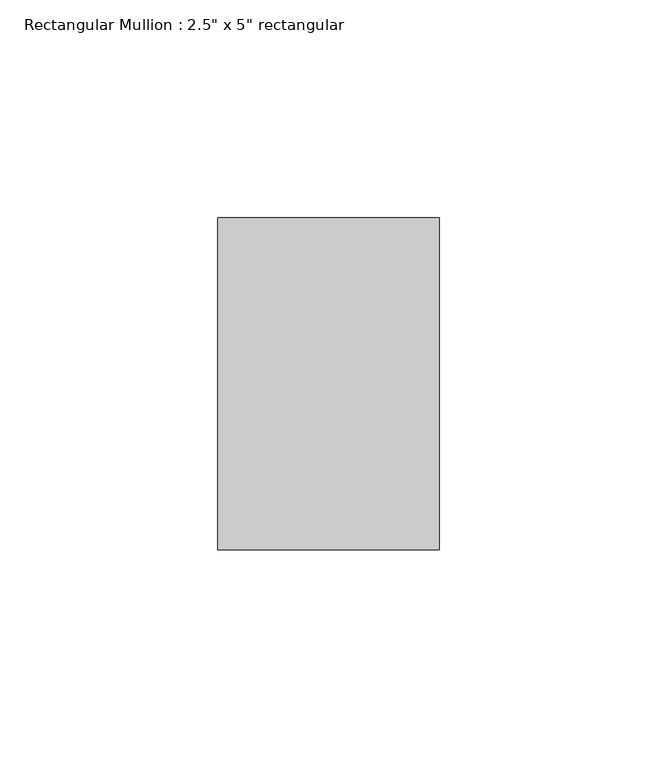
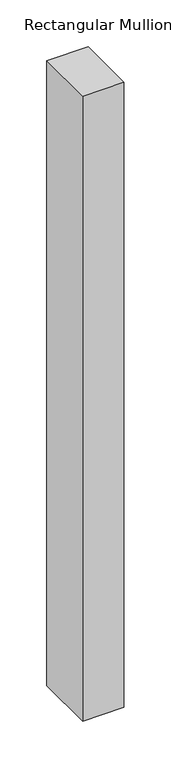
"""IFC4 building model written with IfcOpenShell, lengths in millimetres: member geometry."""

from ifc_helpers import new_model, si_unit, frame, origin, place, context, project, spatial, polyline, outline, extrude, source, transform, mapped, element, save


def member_492a078d(model_context):
    return source(origin(), model_context, "Body", "SweptSolid", [
        extrude(outline(polyline([(0.0, 38.1), (0.0, -38.1), (-50.8, -38.1), (-50.8, 38.1), (0.0, 38.1)])), frame((0.0, 0.0, -812.8), z_axis=(0.0, 0.0, 1.0), x_axis=(1.0, 0.0, 0.0)), (0.0, 0.0, 1.0), 812.8),
    ])


if __name__ == "__main__":
    model = new_model("IFC4")
    model_context = context("Model", 3, world=origin())
    ifc_project = project(units=[si_unit("LENGTHUNIT", "METRE", prefix="MILLI")], contexts=[model_context])
    site = spatial("IfcSite", under=ifc_project)
    building = spatial("IfcBuilding", under=site)
    placement = place(None, origin())
    member_shape = member_492a078d(model_context)
    element("IfcMember", 1, ObjectType="Rectangular Mullion : 2.5\" x 5\" rectangular", at=placement, inside=building, context=model_context, shape_type="MappedRepresentation", body=[
        mapped(member_shape, transform((0.0, 0.0, 0.0), x_axis=(1.0, 0.0, 0.0), y_axis=(0.0, 1.0, 0.0), z_axis=(0.0, 0.0, 1.0))),
    ])
    save(model, "model.ifc")

# Revit data of these elements
# Type "Rectangular Mullion : 2.5\" x 5\" rectangular"
#   built-in parameter 1007304 = 0.25 (stored number, unit not read)
#   built-in parameter 1007301 = 0.0833333 (stored number, unit not read)
#   built-in parameter 1007300 = 0.0833333 (stored number, unit not read)
# Element 1 (IfcMember, "Rectangular Mullion : 2.5\" x 5\" rectangular")
#   Materials on its faces: "Aluminum"
# Materials
#   "Aluminum": class "Metal", colour RGB 244 245 246, transparency 0, Description = "Aluminum 6061", Cost = 0
